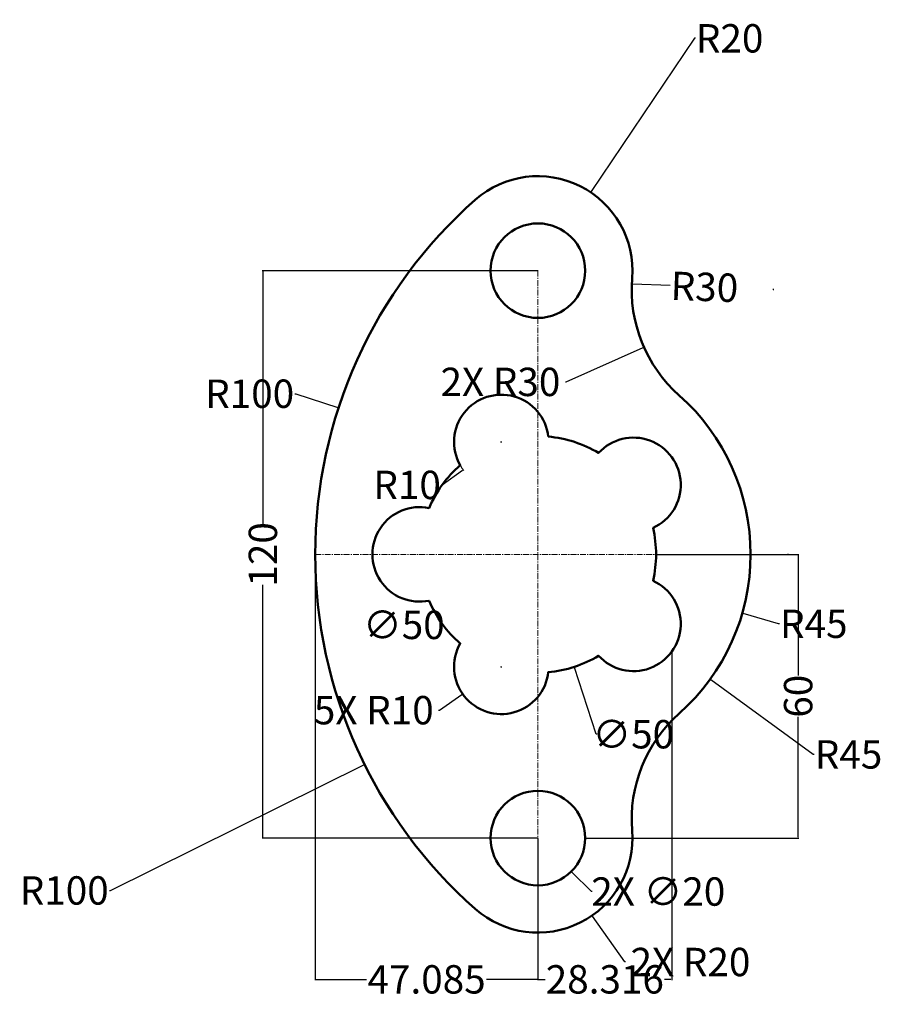
# Model space of a CAD drawing. Units: millimetres. Extents: x -15 to 167, y -34 to 175.
import ezdxf

# ---------------------------------------------------------------- set-up
doc = ezdxf.new("R2010")
doc.units = ezdxf.units.MM
doc.header["$MEASUREMENT"] = 0
doc.linetypes.add('CENTER', pattern=[2, 1.25, -0.25, 0.25, -0.25])
for name, color, linetype, lineweight in [('M-CNTR', 4, 'CENTER', 18), ('M-DIMS', 2, 'Continuous', 25), ('M-OUTL', 7, 'Continuous', 50)]:
    doc.layers.add(name, color=color, linetype=linetype, lineweight=lineweight)
doc.styles.get("Standard").update_dxf_attribs({"font": 'arial.ttf'})
doc.dimstyles.get("Standard").update_dxf_attribs({"dimtxt": 6, "dimasz": 0.18, "dimexe": 0.18, "dimexo": 0.0625, "dimgap": 0.09, "dimtad": 0, "dimtoh": 1, "dimdec": 0, "dimzin": 0, "dimdsep": 46, "dimtxsty": 'Standard', "dimcen": 0.09, "dimadec": 0, "dimazin": 0, "dimtfac": 1, "dimtdec": 0, "dimtofl": 0, "dimtmove": 0, "dimatfit": 3, "dimfxl": 1, "dimtolj": 1, "dimtzin": 0, "dimarcsym": 0})

# ---------------------------------------------------------------- blocks, each defined once
blk = doc.blocks.new('*D1')
at = {"layer": 'Defpoints', "color": 0, "transparency": 16777216}
for p in [(94.18, 121.43), (36.01, 1.43), (94.18, 1.43)]:
    blk.add_point(p, dxfattribs=at)
at = {"layer": 'M-DIMS', "color": 0, "lineweight": -2, "transparency": 16777216}
for p, q in [((94.12, 121.43), (35.83, 121.43)), ((36.01, 121.25), (36.01, 67.86)), ((36.01, 1.61), (36.01, 55)), ((94.12, 1.43), (35.83, 1.43))]:
    blk.add_line(p, q, dxfattribs=at)
at = {"layer": 'M-DIMS', "color": 0, "transparency": 16777216}
for points in [[(35.98, 121.25), (36.04, 121.25), (36.01, 121.43)], [(35.98, 1.61), (36.04, 1.61), (36.01, 1.43)]]:
    blk.add_solid(points, dxfattribs=at)
at = {"layer": 'M-DIMS', "color": 0, "transparency": 16777216, "insert": (36.01, 61.43), "char_height": 6, "attachment_point": 5, "rotation": 90}
blk.add_mtext('\\A1;120', dxfattribs=at)
blk = doc.blocks.new('*D2')
at = {"layer": 'Defpoints', "color": 0, "transparency": 16777216}
for p in [(114.04, 118.57), (144.02, 117.47)]:
    blk.add_point(p, dxfattribs=at)
at = {"layer": 'M-DIMS', "color": 0, "lineweight": -2, "transparency": 16777216}
blk.add_line((122.17, 118.28), (114.22, 118.57), dxfattribs=at)
at = {"layer": 'M-DIMS', "color": 0, "transparency": 16777216}
blk.add_solid([(114.22, 118.6), (114.22, 118.54), (114.04, 118.57)], dxfattribs=at)
at = {"layer": 'M-DIMS', "color": 0, "transparency": 16777216, "insert": (129.42, 118.01), "char_height": 6, "attachment_point": 5, "rotation": 357.892}
blk.add_mtext('\\A1;R30', dxfattribs=at)
blk = doc.blocks.new('*D3')
at = {"layer": 'Defpoints', "color": 0, "transparency": 16777216}
for p in [(94.18, 61.43), (137.42, 48.96)]:
    blk.add_point(p, dxfattribs=at)
at = {"layer": 'M-DIMS', "color": 0, "lineweight": -2, "transparency": 16777216}
for p, q in [((94.09, 61.43), (94.27, 61.43)), ((94.18, 61.34), (94.18, 61.52)), ((145.08, 46.75), (137.59, 48.91)), ((145.26, 46.75), (145.08, 46.75))]:
    blk.add_line(p, q, dxfattribs=at)
at = {"layer": 'M-DIMS', "color": 0, "transparency": 16777216}
blk.add_solid([(137.6, 48.94), (137.58, 48.88), (137.42, 48.96)], dxfattribs=at)
at = {"layer": 'M-DIMS', "color": 0, "transparency": 16777216, "insert": (152.54, 46.75), "char_height": 6, "attachment_point": 5}
blk.add_mtext('\\A1;R45', dxfattribs=at)
blk = doc.blocks.new('*D4')
at = {"layer": 'Defpoints', "color": 0, "transparency": 16777216}
for p in [(86.45, 85.21), (78.36, 79.33)]:
    blk.add_point(p, dxfattribs=at)
at = {"layer": 'M-DIMS', "color": 0, "lineweight": -2, "transparency": 16777216}
for p, q in [((86.36, 85.21), (86.54, 85.21)), ((86.45, 85.12), (86.45, 85.3)), ((73.95, 76.12), (78.22, 79.22)), ((73.77, 76.12), (73.95, 76.12))]:
    blk.add_line(p, q, dxfattribs=at)
blk.add_arc((86.45, 85.21), 10, 209.8951, 217.0313, dxfattribs=at)
at = {"layer": 'M-DIMS', "color": 0, "transparency": 16777216}
blk.add_solid([(78.2, 79.25), (78.23, 79.2), (78.36, 79.33)], dxfattribs=at)
at = {"layer": 'M-DIMS', "color": 0, "transparency": 16777216, "insert": (66.52, 76.12), "char_height": 6, "attachment_point": 5}
blk.add_mtext('\\A1;R10', dxfattribs=at)
blk = doc.blocks.new('*D5')
at = {"layer": 'Defpoints', "color": 0, "transparency": 16777216}
for p in [(114.4, 76.12), (73.95, 46.74)]:
    blk.add_point(p, dxfattribs=at)
at = {"layer": 'M-DIMS', "color": 0, "lineweight": -2, "transparency": 16777216}
for p, q in [((94.09, 61.43), (94.27, 61.43)), ((94.18, 61.34), (94.18, 61.52)), ((73.48, 46.52), (73.66, 46.52)), ((73.66, 46.52), (73.81, 46.63))]:
    blk.add_line(p, q, dxfattribs=at)
at = {"layer": 'M-DIMS', "color": 0, "transparency": 16777216}
blk.add_solid([(73.79, 46.65), (73.82, 46.61), (73.95, 46.74)], dxfattribs=at)
at = {"layer": 'M-DIMS', "color": 0, "transparency": 16777216, "insert": (65.84, 46.52), "char_height": 6, "attachment_point": 5}
blk.add_mtext('\\A1;∅50', dxfattribs=at)
blk = doc.blocks.new('*D6')
at = {"layer": 'Defpoints', "color": 0, "transparency": 16777216}
for p in [(52.03, 92.46), (147.09, 61.43)]:
    blk.add_point(p, dxfattribs=at)
at = {"layer": 'M-DIMS', "color": 0, "lineweight": -2, "transparency": 16777216}
for p, q in [((42.8, 95.41), (42.98, 95.41)), ((42.98, 95.41), (51.86, 92.52)), ((147, 61.43), (147.18, 61.43)), ((147.09, 61.34), (147.09, 61.52))]:
    blk.add_line(p, q, dxfattribs=at)
at = {"layer": 'M-DIMS', "color": 0, "transparency": 16777216}
blk.add_solid([(51.87, 92.54), (51.85, 92.49), (52.03, 92.46)], dxfattribs=at)
at = {"layer": 'M-DIMS', "color": 0, "transparency": 16777216, "insert": (33.22, 95.41), "char_height": 6, "attachment_point": 5}
blk.add_mtext('\\A1;R100', dxfattribs=at)
blk = doc.blocks.new('*D7')
at = {"layer": 'Defpoints', "color": 0, "transparency": 16777216}
for p in [(105.36, 138.01), (94.18, 121.43)]:
    blk.add_point(p, dxfattribs=at)
at = {"layer": 'M-DIMS', "color": 0, "lineweight": -2, "transparency": 16777216}
for p, q in [((127.31, 170.57), (105.46, 138.16)), ((127.49, 170.57), (127.31, 170.57)), ((94.09, 121.43), (94.27, 121.43)), ((94.18, 121.34), (94.18, 121.52))]:
    blk.add_line(p, q, dxfattribs=at)
at = {"layer": 'M-DIMS', "color": 0, "transparency": 16777216}
blk.add_solid([(105.43, 138.18), (105.48, 138.15), (105.36, 138.01)], dxfattribs=at)
at = {"layer": 'M-DIMS', "color": 0, "transparency": 16777216, "insert": (134.74, 170.57), "char_height": 6, "attachment_point": 5}
blk.add_mtext('\\A1;R20', dxfattribs=at)
blk = doc.blocks.new('MOUNT-HOLE-D20')
blk.add_circle((0, 0), 10)
blk = doc.blocks.new('*D9')
at = {"layer": 'Defpoints', "color": 0, "transparency": 16777216}
for p in [(47.09, 61.43), (94.18, 1.43), (94.18, -28.45)]:
    blk.add_point(p, dxfattribs=at)
at = {"layer": 'M-DIMS', "color": 0, "lineweight": -2, "transparency": 16777216}
for p, q in [((47.09, 61.37), (47.09, -28.63)), ((94.18, 1.37), (94.18, -28.63)), ((47.27, -28.45), (57.95, -28.45)), ((94, -28.45), (83.32, -28.45))]:
    blk.add_line(p, q, dxfattribs=at)
at = {"layer": 'M-DIMS', "color": 0, "transparency": 16777216}
for points in [[(47.27, -28.42), (47.27, -28.48), (47.09, -28.45)], [(94, -28.42), (94, -28.48), (94.18, -28.45)]]:
    blk.add_solid(points, dxfattribs=at)
at = {"layer": 'M-DIMS', "color": 0, "transparency": 16777216, "insert": (70.64, -28.45), "char_height": 6, "attachment_point": 5}
blk.add_mtext('\\A1;47.085', dxfattribs=at)
blk = doc.blocks.new('*D10')
at = {"layer": 'Defpoints', "color": 0, "transparency": 16777216}
for p in [(119.18, 61.43), (104.18, 1.43), (149.23, 1.43)]:
    blk.add_point(p, dxfattribs=at)
at = {"layer": 'M-DIMS', "color": 0, "lineweight": -2, "transparency": 16777216}
for p, q in [((119.24, 61.43), (149.41, 61.43)), ((149.23, 61.25), (149.23, 35.82)), ((149.23, 1.61), (149.23, 27.04)), ((104.24, 1.43), (149.41, 1.43))]:
    blk.add_line(p, q, dxfattribs=at)
at = {"layer": 'M-DIMS', "color": 0, "transparency": 16777216}
for points in [[(149.2, 61.25), (149.26, 61.25), (149.23, 61.43)], [(149.2, 1.61), (149.26, 1.61), (149.23, 1.43)]]:
    blk.add_solid(points, dxfattribs=at)
at = {"layer": 'M-DIMS', "color": 0, "transparency": 16777216, "insert": (149.23, 31.43), "char_height": 6, "attachment_point": 5, "rotation": 90}
blk.add_mtext('\\A1;60', dxfattribs=at)
blk = doc.blocks.new('*D11')
at = {"layer": 'Defpoints', "color": 0, "transparency": 16777216}
for p in [(122.49, 40.86), (94.18, 1.43), (122.49, -28.45)]:
    blk.add_point(p, dxfattribs=at)
at = {"layer": 'M-DIMS', "color": 0, "lineweight": -2, "transparency": 16777216}
for p, q in [((122.49, 40.79), (122.49, -28.63)), ((94.18, 1.37), (94.18, -28.63)), ((94.36, -28.45), (95.74, -28.45)), ((122.31, -28.45), (120.93, -28.45))]:
    blk.add_line(p, q, dxfattribs=at)
at = {"layer": 'M-DIMS', "color": 0, "transparency": 16777216}
for points in [[(94.36, -28.42), (94.36, -28.48), (94.18, -28.45)], [(122.31, -28.42), (122.31, -28.48), (122.49, -28.45)]]:
    blk.add_solid(points, dxfattribs=at)
at = {"layer": 'M-DIMS', "color": 0, "transparency": 16777216, "insert": (108.34, -28.45), "char_height": 6, "attachment_point": 5}
blk.add_mtext('\\A1;28.316', dxfattribs=at)
blk = doc.blocks.new('*D12')
at = {"layer": 'Defpoints', "color": 0, "transparency": 16777216}
for p in [(87.11, 8.5), (101.25, -5.64)]:
    blk.add_point(p, dxfattribs=at)
at = {"layer": 'M-DIMS', "color": 0, "lineweight": -2, "transparency": 16777216}
for p, q in [((94.09, 1.43), (94.27, 1.43)), ((94.18, 1.34), (94.18, 1.52)), ((105.49, -9.88), (101.38, -5.77)), ((105.67, -9.88), (105.49, -9.88))]:
    blk.add_line(p, q, dxfattribs=at)
at = {"layer": 'M-DIMS', "color": 0, "transparency": 16777216}
blk.add_solid([(101.4, -5.75), (101.36, -5.79), (101.25, -5.64)], dxfattribs=at)
at = {"layer": 'M-DIMS', "color": 0, "transparency": 16777216, "insert": (119.65, -9.88), "char_height": 6, "attachment_point": 5}
blk.add_mtext('\\A1;2X ∅20', dxfattribs=at)
blk = doc.blocks.new('*D13')
at = {"layer": 'Defpoints', "color": 0, "transparency": 16777216}
for p in [(94.18, 1.43), (105.65, -14.95)]:
    blk.add_point(p, dxfattribs=at)
at = {"layer": 'M-DIMS', "color": 0, "lineweight": -2, "transparency": 16777216}
for p, q in [((94.09, 1.43), (94.27, 1.43)), ((94.18, 1.34), (94.18, 1.52)), ((112.54, -24.78), (105.75, -15.1)), ((112.72, -24.78), (112.54, -24.78))]:
    blk.add_line(p, q, dxfattribs=at)
at = {"layer": 'M-DIMS', "color": 0, "transparency": 16777216}
blk.add_solid([(105.78, -15.08), (105.73, -15.12), (105.65, -14.95)], dxfattribs=at)
at = {"layer": 'M-DIMS', "color": 0, "transparency": 16777216, "insert": (126.46, -24.78), "char_height": 6, "attachment_point": 5}
blk.add_mtext('\\A1;2X R20', dxfattribs=at)
blk = doc.blocks.new('*D14')
at = {"layer": 'Defpoints', "color": 0, "transparency": 16777216}
for p in [(94.18, 61.43), (130.59, 34.98)]:
    blk.add_point(p, dxfattribs=at)
at = {"layer": 'M-DIMS', "color": 0, "lineweight": -2, "transparency": 16777216}
for p, q in [((94.09, 61.43), (94.27, 61.43)), ((94.18, 61.34), (94.18, 61.52)), ((152.43, 19.12), (130.73, 34.88)), ((152.61, 19.12), (152.43, 19.12))]:
    blk.add_line(p, q, dxfattribs=at)
at = {"layer": 'M-DIMS', "color": 0, "transparency": 16777216}
blk.add_solid([(130.75, 34.9), (130.71, 34.85), (130.59, 34.98)], dxfattribs=at)
at = {"layer": 'M-DIMS', "color": 0, "transparency": 16777216, "insert": (159.89, 19.12), "char_height": 6, "attachment_point": 5}
blk.add_mtext('\\A1;R45', dxfattribs=at)
blk = doc.blocks.new('*D15')
at = {"layer": 'Defpoints', "color": 0, "transparency": 16777216}
for p in [(86.45, 37.65), (78.26, 31.92)]:
    blk.add_point(p, dxfattribs=at)
at = {"layer": 'M-DIMS', "color": 0, "lineweight": -2, "transparency": 16777216}
for p, q in [((86.36, 37.65), (86.54, 37.65)), ((86.45, 37.56), (86.45, 37.74)), ((73.34, 28.48), (78.11, 31.82)), ((73.16, 28.48), (73.34, 28.48))]:
    blk.add_line(p, q, dxfattribs=at)
at = {"layer": 'M-DIMS', "color": 0, "transparency": 16777216}
blk.add_solid([(78.09, 31.84), (78.13, 31.79), (78.26, 31.92)], dxfattribs=at)
at = {"layer": 'M-DIMS', "color": 0, "transparency": 16777216, "insert": (59.47, 28.48), "char_height": 6, "attachment_point": 5}
blk.add_mtext('\\A1;5X R10', dxfattribs=at)
blk = doc.blocks.new('*D16')
at = {"layer": 'Defpoints', "color": 0, "transparency": 16777216}
for p in [(86.45, 85.21), (101.9, 37.65)]:
    blk.add_point(p, dxfattribs=at)
at = {"layer": 'M-DIMS', "color": 0, "lineweight": -2, "transparency": 16777216}
for p, q in [((94.09, 61.43), (94.27, 61.43)), ((94.18, 61.34), (94.18, 61.52)), ((106.54, 23.39), (101.96, 37.48)), ((106.72, 23.39), (106.54, 23.39))]:
    blk.add_line(p, q, dxfattribs=at)
at = {"layer": 'M-DIMS', "color": 0, "transparency": 16777216}
blk.add_solid([(101.99, 37.49), (101.93, 37.47), (101.9, 37.65)], dxfattribs=at)
at = {"layer": 'M-DIMS', "color": 0, "transparency": 16777216, "insert": (114.36, 23.39), "char_height": 6, "attachment_point": 5}
blk.add_mtext('\\A1;∅50', dxfattribs=at)
blk = doc.blocks.new('*D17')
at = {"layer": 'Defpoints', "color": 0, "transparency": 16777216}
for p in [(144.02, 117.47), (116.63, 105.24)]:
    blk.add_point(p, dxfattribs=at)
at = {"layer": 'M-DIMS', "color": 0, "lineweight": -2, "transparency": 16777216}
for p, q in [((143.93, 117.47), (144.11, 117.47)), ((144.02, 117.38), (144.02, 117.56)), ((100.19, 97.91), (116.46, 105.17)), ((100.01, 97.91), (100.19, 97.91))]:
    blk.add_line(p, q, dxfattribs=at)
at = {"layer": 'M-DIMS', "color": 0, "transparency": 16777216}
blk.add_solid([(116.45, 105.2), (116.47, 105.14), (116.63, 105.24)], dxfattribs=at)
at = {"layer": 'M-DIMS', "color": 0, "transparency": 16777216, "insert": (86.26, 97.91), "char_height": 6, "attachment_point": 5}
blk.add_mtext('\\A1;2X R30', dxfattribs=at)
blk = doc.blocks.new('*D18')
at = {"layer": 'Defpoints', "color": 0, "transparency": 16777216}
for p in [(147.09, 61.43), (57.5, 17.01)]:
    blk.add_point(p, dxfattribs=at)
at = {"layer": 'M-DIMS', "color": 0, "lineweight": -2, "transparency": 16777216}
for p, q in [((147, 61.43), (147.18, 61.43)), ((147.09, 61.34), (147.09, 61.52)), ((3.75, -9.65), (57.34, 16.93)), ((3.57, -9.65), (3.75, -9.65))]:
    blk.add_line(p, q, dxfattribs=at)
at = {"layer": 'M-DIMS', "color": 0, "transparency": 16777216}
blk.add_solid([(57.33, 16.95), (57.35, 16.9), (57.5, 17.01)], dxfattribs=at)
at = {"layer": 'M-DIMS', "color": 0, "transparency": 16777216, "insert": (-6.01, -9.65), "char_height": 6, "attachment_point": 5}
blk.add_mtext('\\A1;R100', dxfattribs=at)

msp = doc.modelspace()

# ---------------------------------------------------------------- linework, layer by layer
at = {"layer": 'M-CNTR'}
msp.add_line((47.0926, 61.4298), (139.1775, 61.4298), dxfattribs=at)
msp.add_lwpolyline([(94.1775, 121.4298), (94.1775, 61.4298), (94.1775, 1.4298)], dxfattribs=at)
at = {"layer": 'M-OUTL'}
for points in [[(114.1148, 119.8465, 0.2349668), (124.0834, 95.0548, -0.4488969), (124.0834, 27.8048, 0.2349668), (114.1148, 3.0131, -0.67419298), (80.9488, -13.5702, -0.45141623), (80.9488, 136.4298, -0.67419298)], [(96.3886, 86.3318, 1.22474487), (77.7517, 80.2764, 0.11328223), (71.1775, 71.2278, 1.22474487), (71.1775, 51.6318, 0.11328223), (77.7517, 42.5832, 1.22474487), (96.3886, 36.5278, 0.11328223), (107.0258, 39.984, 1.22474487), (118.544, 55.8374, 0.11328223), (118.544, 67.0221, 1.22474487), (107.0258, 82.8756, 0.11328223)]]:
    msp.add_lwpolyline(points, format="xyb", close=True, dxfattribs=at)

# ---------------------------------------------------------------- block references
for p in [(94.1775, 121.4298), (94.1775, 1.4298)]:
    msp.add_blockref('MOUNT-HOLE-D20', p, dxfattribs=at)

# ---------------------------------------------------------------- dimensions: what is measured, and where the dimension line sits
at = {"layer": 'M-DIMS'}
for center, mpoint, override, picture, middle in [((94.1775, 121.4298), (105.3584, 138.0125), {"dimclrd": 0, "dimclre": 0, "dimclrt": 0}, '*D7', (134.741, 170.5736)), ((144.0206, 117.4715), (114.0409, 118.5749), {"dimclrd": 0, "dimclre": 0, "dimclrt": 0}, '*D2', (129.4161, 118.009)), ((147.0926, 61.4298), (52.0287, 92.4598), {"dimclrd": 0, "dimclre": 0, "dimclrt": 0}, '*D6', (33.2168, 95.4148)), ((86.4521, 85.2062), (78.3619, 79.3284), {"dimclrd": 0, "dimclre": 0, "dimclrt": 0}, '*D4', (66.5239, 76.1244)), ((147.0926, 61.4298), (57.5018, 17.0058), {"dimdec": 0, "dimlfac": 1, "dimrnd": 0, "dimzin": 0, "dimdsep": 46, "dimlunit": 2}, '*D18', (-6.0118, -9.6485)), ((94.1775, 61.4298), (137.4155, 48.9606), {"dimclrd": 0, "dimclre": 0, "dimclrt": 0}, '*D3', (152.5408, 46.7503)), ((94.1775, 61.4298), (130.586, 34.9831), {"dimdec": 0, "dimlfac": 1, "dimrnd": 0, "dimzin": 0, "dimdsep": 46, "dimlunit": 2}, '*D14', (159.892, 19.1151))]:
    dim = msp.add_radius_dim(center=center, mpoint=mpoint, dimstyle='Standard', override=override, dxfattribs=at)
    dim.commit()
    dim.dimension.update_dxf_attribs({"geometry": picture, "text_midpoint": middle, "dimtype": 164})
for base, p1, p2, override, picture, middle in [((36.0143, 1.4298), (94.1775, 121.4298), (94.1775, 1.4298), {"dimclrd": 0, "dimclre": 0, "dimclrt": 0}, '*D1', (36.0143, 61.4298)), ((149.2275, 1.4298), (119.1775, 61.4298), (104.1775, 1.4298), {"dimdec": 0, "dimlfac": 1, "dimrnd": 0, "dimzin": 0, "dimdsep": 46, "dimlunit": 2}, '*D10', (149.2275, 31.4298))]:
    dim = msp.add_linear_dim(base=base, p1=p1, p2=p2, angle=90, dimstyle='Standard', override=override, dxfattribs=at)
    dim.commit()
    dim.dimension.update_dxf_attribs({"geometry": picture, "text_midpoint": middle})
for center, mpoint, text, picture, middle in [((144.0206, 117.4715), (116.626, 105.2429), '2X <>', '*D17', (86.2638, 97.9058)), ((86.4521, 37.6534), (78.2593, 31.9195), '5X <>', '*D15', (59.4692, 28.4792)), ((94.1775, 1.4298), (105.6512, -14.9517), '2X <>', '*D13', (126.461, -24.7807))]:
    dim = msp.add_radius_dim(center=center, mpoint=mpoint, text=text, dimstyle='Standard', override={"dimdec": 0, "dimlfac": 1, "dimrnd": 0, "dimzin": 0, "dimdsep": 46, "dimlunit": 2}, dxfattribs=at)
    dim.commit()
    dim.dimension.update_dxf_attribs({"geometry": picture, "text_midpoint": middle, "dimtype": 164})
dim = msp.add_diameter_dim_2p(p1=(86.4522, 85.2062), p2=(101.9029, 37.6534), dimstyle='Standard', override={"dimdec": 0, "dimlfac": 1, "dimrnd": 0, "dimzin": 0, "dimdsep": 46, "dimlunit": 2}, dxfattribs=at)
dim.commit()
dim.dimension.update_dxf_attribs({"geometry": '*D16', "text_midpoint": (114.3593, 23.3875), "dimtype": 163})
dim = msp.add_diameter_dim_2p(p1=(114.403, 76.1244), p2=(73.9521, 46.7352), dimstyle='Standard', override={"dimclrd": 0, "dimclre": 0, "dimclrt": 0}, dxfattribs=at)
dim.commit()
dim.dimension.update_dxf_attribs({"geometry": '*D5', "text_midpoint": (65.8397, 46.5236)})
for base, p1, p2, picture, middle in [((94.1775, -28.4526), (47.0926, 61.4298), (94.1775, 1.4298), '*D9', (70.635, -28.4526)), ((122.4931, -28.4526), (94.1775, 1.4298), (122.4931, 40.8573), '*D11', (108.3353, -28.4526))]:
    dim = msp.add_linear_dim(base=base, p1=p1, p2=p2, dimstyle='Standard', override={"dimdec": 3, "dimlfac": 1, "dimrnd": 0, "dimzin": 0, "dimdsep": 46, "dimlunit": 2}, dxfattribs=at)
    dim.commit()
    dim.dimension.update_dxf_attribs({"geometry": picture, "text_midpoint": middle})
dim = msp.add_diameter_dim_2p(p1=(87.1051, 8.4995), p2=(101.2499, -5.6399), text='2X <>', dimstyle='Standard', override={"dimdec": 0, "dimlfac": 1, "dimrnd": 0, "dimzin": 0, "dimdsep": 46, "dimlunit": 2}, dxfattribs=at)
dim.commit()
dim.dimension.update_dxf_attribs({"geometry": '*D12', "text_midpoint": (119.6522, -9.8818), "dimtype": 163})

doc.saveas('drawing.dxf')
